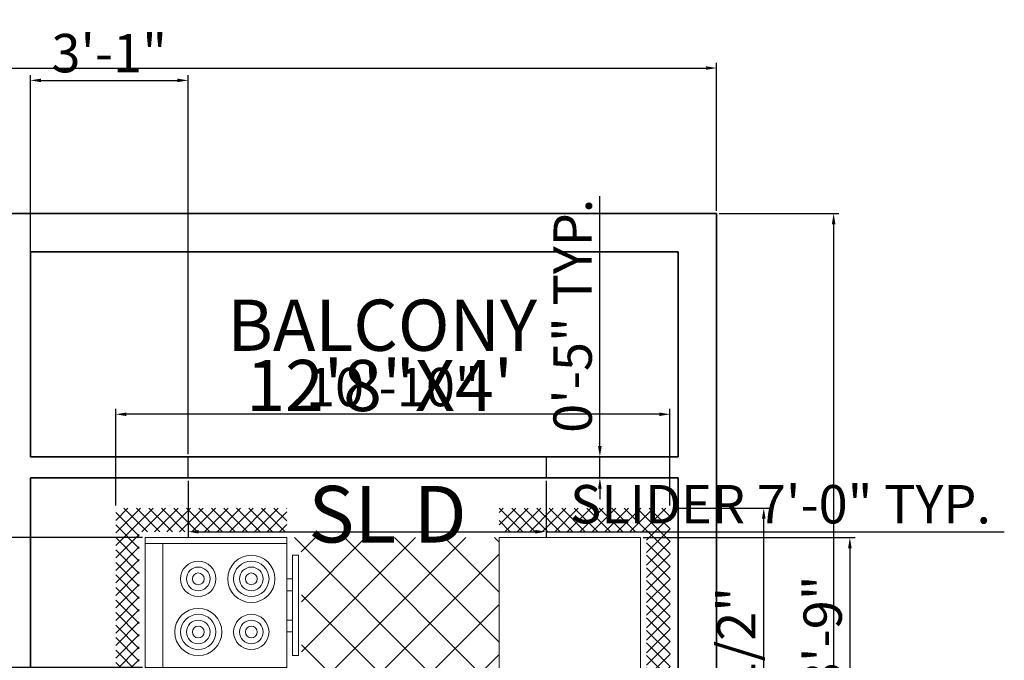
# Model space of a CAD drawing. Units: inches. Extents: x 3542 to 4275, y 1005 to 1722.
# Tile 6 of 6: x 4018 to 4249, y 1568 to 1718. Entities that reach past the tile are written whole.
import ezdxf

# ---------------------------------------------------------------- set-up
doc = ezdxf.new("R2010")
doc.units = ezdxf.units.IN
doc.layers.get('0').update_dxf_attribs({"color": 211})
for name, color, linetype, lineweight in [('A-ANNO-DIMS', 2, 'Continuous', 18), ('A-ANNO-TEXT', 7, 'Continuous', 18), ('A-AREA-IDEN', 7, 'Continuous', 25), ('A-DOOR', 3, 'Continuous', 25), ('A-FLOR-FIXT', 9, 'Continuous', 18), ('wall', 7, 'Continuous', 35)]:
    doc.layers.add(name, color=color, linetype=linetype, lineweight=lineweight)
doc.styles.get("Standard").update_dxf_attribs({"font": 'arial.ttf'})
doc.dimstyles.new('ISO-25', dxfattribs={"dimtxt": 9, "dimasz": 2.5, "dimexe": 1.25, "dimexo": 0.625, "dimtad": 1, "dimdec": 1, "dimlunit": 4, "dimtxsty": 'Standard', "dimcen": 2.5, "dimadec": 0, "dimazin": 0, "dimtfac": 1, "dimtdec": 1, "dimtmove": 0, "dimatfit": 3, "dimfxl": 1, "dimarcsym": 0})

# ---------------------------------------------------------------- blocks, each defined once
blk = doc.blocks.new('Kitchen Layout - 7 x 8 ft')
for p, q in [((-5, 81.32), (2.68, 89)), ((-5, 83.44), (0.56, 89)), ((-5, 85.56), (-1.56, 89)), ((-5, 87.68), (-3.68, 89)), ((-1, 84.97), (-5, 88.97)), ((1.09, 85), (-2.91, 89)), ((3.21, 85), (-0.79, 89)), ((0.81, 85), (4.81, 89)), ((5.34, 85), (1.34, 89)), ((2.93, 85), (6.93, 89)), ((7.46, 85), (3.46, 89)), ((5.05, 85), (9.05, 89)), ((9.58, 85), (5.58, 89)), ((7.17, 85), (11.17, 89)), ((11.7, 85), (7.7, 89)), ((9.29, 85), (13.29, 89)), ((13.82, 85), (9.82, 89)), ((11.41, 85), (15.41, 89)), ((15.94, 85), (11.94, 89)), ((13.53, 85), (17.53, 89)), ((18.06, 85), (14.06, 89)), ((15.65, 85), (19.65, 89)), ((20.18, 85), (16.18, 89)), ((17.78, 85), (21.78, 89)), ((22.31, 85), (18.31, 89)), ((19.9, 85), (23.9, 89)), ((24.43, 85), (20.43, 89)), ((22.02, 85), (26.02, 89)), ((26.55, 85), (22.55, 89)), ((24.14, 85), (28.14, 89)), ((28.67, 85), (24.67, 89)), ((26.26, 85), (30.26, 89)), ((30.79, 85), (26.79, 89)), ((28.38, 85), (32.38, 89)), ((32.91, 85), (28.91, 89)), ((30.5, 85), (34.5, 89)), ((35.03, 85), (31.03, 89)), ((32.63, 85), (36.63, 89)), ((37.16, 85), (33.16, 89)), ((34.75, 85), (38.75, 89)), ((39.28, 85), (35.28, 89)), ((36.87, 85), (40.87, 89)), ((41.4, 85), (37.4, 89)), ((38.99, 85), (42.99, 89)), ((43.52, 85), (39.52, 89)), ((41.11, 85), (45.11, 89)), ((45.64, 85), (41.64, 89)), ((43.23, 85), (47.23, 89)), ((47.76, 85), (43.76, 89)), ((45.35, 85), (49.35, 89)), ((49.88, 85), (45.88, 89)), ((47.47, 85), (51.47, 89)), ((52, 85), (48, 89)), ((49.6, 85), (53.6, 89)), ((54.13, 85), (50.13, 89)), ((51.72, 85), (55.72, 89)), ((56.25, 85), (52.25, 89)), ((53.84, 85), (57.84, 89)), ((58.37, 85), (54.37, 89)), ((55.96, 85), (59.96, 89)), ((60.49, 85), (56.49, 89)), ((58.08, 85), (62.08, 89)), ((62.61, 85), (58.61, 89)), ((60.2, 85), (64.2, 89)), ((64.73, 85), (60.73, 89)), ((62.32, 85), (66.32, 89)), ((66.85, 85), (62.85, 89)), ((64.45, 85), (68.45, 89)), ((68.97, 85), (64.97, 89)), ((66.57, 85), (70.57, 89)), ((71.1, 85), (67.1, 89)), ((68.69, 85), (72.69, 89)), ((73.22, 85), (69.22, 89)), ((70.81, 85), (74.81, 89)), ((75.34, 85), (71.34, 89)), ((72.93, 85), (76.93, 89)), ((77.46, 85), (73.46, 89)), ((75.05, 85), (79.05, 89)), ((79.58, 85), (75.58, 89)), ((77.17, 85), (81.17, 89)), ((81.7, 85), (77.7, 89)), ((79.29, 85), (83.29, 89)), ((83.82, 85), (79.82, 89)), ((81.42, 85), (85.42, 89)), ((85.95, 85), (81.95, 89)), ((83.54, 85), (87.54, 89)), ((88.07, 85), (84.07, 89)), ((85.66, 85), (89.66, 89)), ((90.19, 85), (86.19, 89)), ((87.78, 85), (91.78, 89)), ((92.31, 85), (88.31, 89)), ((89.9, 85), (93.9, 89)), ((94.43, 85), (90.43, 89)), ((92.02, 85), (96.02, 89)), ((96.55, 85), (92.55, 89)), ((94.14, 85), (98.14, 89)), ((101, 82.67), (94.67, 89)), ((96.27, 85), (100.27, 89)), ((101, 84.79), (96.79, 89)), ((101, 86.92), (98.92, 89)), ((-1, 82.85), (-5, 86.85)), ((97, 83.61), (101, 87.61)), ((97, 81.49), (101, 85.49)), ((-1, 80.73), (-5, 84.73)), ((34, 84), (96, 84)), ((34, 60), (34, 84)), ((96, 84), (96, 60)), ((101, 80.55), (97, 84.55)), ((-5, 79.19), (-1, 83.19)), ((-1, 78.61), (-5, 82.61)), ((97, 79.37), (101, 83.37)), ((101, 78.43), (97, 82.43)), ((-5, 77.07), (-1, 81.07)), ((-1, 76.49), (-5, 80.49)), ((74, 81), (95, 81)), ((97, 77.25), (101, 81.25)), ((101, 76.31), (97, 80.31)), ((-5, 74.95), (-1, 78.95)), ((97, 75.13), (101, 79.13)), ((-1, 74.36), (-5, 78.36)), ((-5, 72.83), (-1, 76.83)), ((101, 74.19), (97, 78.19)), ((97, 73.01), (101, 77.01)), ((-1, 72.24), (-5, 76.24)), ((101, 72.07), (97, 76.07)), ((-5, 70.71), (-1, 74.71)), ((-1, 70.12), (-5, 74.12)), ((97, 70.89), (101, 74.89)), ((101, 69.95), (97, 73.95)), ((-5, 68.59), (-1, 72.59)), ((-1, 68), (-5, 72)), ((97, 68.76), (101, 72.76)), ((101, 67.82), (97, 71.82)), ((-5, 66.47), (-1, 70.47)), ((97, 66.64), (101, 70.64)), ((-1, 65.88), (-5, 69.88)), ((101, 65.7), (97, 69.7)), ((97, 64.52), (101, 68.52)), ((-5, 64.35), (-1, 68.35)), ((-1, 63.76), (-5, 67.76)), ((101, 63.58), (97, 67.58)), ((-5, 62.22), (-1, 66.22)), ((-1, 61.64), (-5, 65.64)), ((97, 62.4), (101, 66.4)), ((101, 61.46), (97, 65.46)), ((-5, 60.1), (-1, 64.1)), ((-1, 59.52), (-5, 63.52)), ((97, 60.28), (101, 64.28)), ((-5, 57.98), (-1, 61.98)), ((100.34, 60), (97, 63.34)), ((98.84, 60), (101, 62.16)), ((-1, 57.39), (-5, 61.39)), ((98.22, 60), (97, 61.22)), ((-1.73, 56), (-5, 59.27)), ((-4.86, 56), (-1, 59.86)), ((10.4, 24), (45.9, 59.5)), ((18.88, 24), (54.38, 59.5)), ((27.37, 24), (62.87, 59.5)), ((33.03, 55.11), (37.41, 59.5)), ((96, 60), (34, 60)), ((35.85, 24), (71.35, 59.5)), ((76.2, 24), (40.7, 59.5)), ((84.68, 24), (49.18, 59.5)), ((93.17, 24), (57.67, 59.5)), ((61.31, 24), (96, 58.69)), ((96, 29.65), (66.15, 59.5)), ((80, 60), (80, 59)), ((82, 59), (82, 60)), ((87, 59), (87, 60)), ((89, 60), (89, 59)), ((100.96, 60), (101, 60.04)), ((-3.85, 56), (-5, 57.15)), ((-2.74, 56), (-1, 57.74)), ((0, 57), (33, 57)), ((67.71, 24), (33.68, 58.04)), ((44.34, 24), (77.84, 57.5)), ((52.82, 24), (86.32, 57.5)), ((96, 38.14), (76.64, 57.5)), ((96, 46.63), (85.13, 57.5)), ((96, 55.11), (93.57, 57.54)), ((31, 55), (31, 56)), ((32, 56), (32, 55)), ((0, 30.57), (24.43, 55)), ((0, 39.06), (15.94, 55)), ((0, 47.54), (7.46, 55)), ((1.91, 24), (32.91, 55)), ((33.77, 24), (2.77, 55)), ((42.26, 24), (11.26, 55)), ((50.74, 24), (19.74, 55)), ((59.23, 24), (28.23, 55)), ((32, 55), (31, 55)), ((69.79, 24), (96, 50.21)), ((25.29, 24), (0, 49.29)), ((16.8, 24), (0, 40.8)), ((78.28, 24), (96, 41.72)), ((8.32, 24), (0, 32.32)), ((86.76, 24), (96, 33.24)), ((-5, 21.92), (-2.92, 24)), ((-5, 19.8), (-1, 23.8)), ((-1, 21.33), (-3.67, 24)), ((-1, 23.45), (-1.55, 24)), ((0, 24), (96, 24)), ((0, 0), (0, 24)), ((95.25, 24), (96, 24.75)), ((96, 24), (96, 0)), ((97, 22.1), (98.9, 24)), ((97, 19.97), (101, 23.97)), ((101, 21.16), (98.16, 24)), ((101, 23.28), (100.28, 24)), ((-1, 19.21), (-5, 23.21)), ((101, 19.03), (97, 23.03)), ((97, 17.85), (101, 21.85)), ((-5, 17.68), (-1, 21.68)), ((-1, 17.09), (-5, 21.09)), ((101, 16.91), (97, 20.91)), ((-5, 15.55), (-1, 19.55)), ((-1, 14.97), (-5, 18.97)), ((47.25, 6.5), (47.25, 18.5)), ((48.75, 18.5), (48.75, 6.5)), ((97, 15.73), (101, 19.73)), ((101, 14.79), (97, 18.79)), ((-5, 13.43), (-1, 17.43)), ((-1, 12.85), (-5, 16.85)), ((97, 13.61), (101, 17.61)), ((-5, 11.31), (-1, 15.31)), ((101, 12.67), (97, 16.67)), ((97, 11.49), (101, 15.49)), ((-1, 10.73), (-5, 14.73)), ((101, 10.55), (97, 14.55)), ((97, 9.37), (101, 13.37)), ((-5, 9.19), (-1, 13.19)), ((-1, 8.6), (-5, 12.6)), ((101, 8.43), (97, 12.43)), ((-5, 7.07), (-1, 11.07)), ((-1, 6.48), (-5, 10.48)), ((97, 7.25), (101, 11.25)), ((101, 6.31), (97, 10.31)), ((-5, 4.95), (-1, 8.95)), ((-1, 4.36), (-5, 8.36)), ((97, 5.12), (101, 9.12)), ((-5, 2.83), (-1, 6.83)), ((101, 4.18), (97, 8.18)), ((97, 3), (101, 7)), ((-1, 2.24), (-5, 6.24)), ((101, 2.06), (97, 6.06)), ((-5, 0.71), (-1, 4.71)), ((-1, 0.12), (-5, 4.12)), ((64, 4), (32, 4)), ((97, 0.88), (101, 4.88)), ((101, -0.06), (97, 3.94)), ((-5, -1.42), (-1, 2.58)), ((2, -5), (-5, 2)), ((93.24, -5), (101, 2.76)), ((101, -2.18), (97, 1.82)), ((-5, -3.54), (-1, 0.46)), ((96, 0), (0, 0)), ((95.36, -5), (101, 0.64)), ((-0.12, -5), (-5, -0.12)), ((-4.34, -5), (-0.34, -1)), ((-2.22, -5), (1.78, -1)), ((-0.1, -5), (3.9, -1)), ((4.12, -5), (0.12, -1)), ((2.02, -5), (6.02, -1)), ((6.24, -5), (2.24, -1)), ((4.14, -5), (8.14, -1)), ((8.36, -5), (4.36, -1)), ((6.27, -5), (10.27, -1)), ((10.48, -5), (6.48, -1)), ((8.39, -5), (12.39, -1)), ((12.6, -5), (8.6, -1)), ((10.51, -5), (14.51, -1)), ((14.73, -5), (10.73, -1)), ((12.63, -5), (16.63, -1)), ((16.85, -5), (12.85, -1)), ((14.75, -5), (18.75, -1)), ((18.97, -5), (14.97, -1)), ((16.87, -5), (20.87, -1)), ((21.09, -5), (17.09, -1)), ((18.99, -5), (22.99, -1)), ((23.21, -5), (19.21, -1)), ((21.11, -5), (25.11, -1)), ((25.33, -5), (21.33, -1)), ((23.24, -5), (27.24, -1)), ((27.45, -5), (23.45, -1)), ((25.36, -5), (29.36, -1)), ((29.57, -5), (25.57, -1)), ((30, -3.3), (27.7, -1)), ((30, -1.18), (29.82, -1)), ((66, -2.54), (67.54, -1)), ((66, -4.66), (69.66, -1)), ((69.88, -5), (66, -1.12)), ((67.78, -5), (71.78, -1)), ((72, -5), (68, -1)), ((69.9, -5), (73.9, -1)), ((74.12, -5), (70.12, -1)), ((72.03, -5), (76.03, -1)), ((76.24, -5), (72.24, -1)), ((74.15, -5), (78.15, -1)), ((78.36, -5), (74.36, -1)), ((76.27, -5), (80.27, -1)), ((80.49, -5), (76.49, -1)), ((78.39, -5), (82.39, -1)), ((82.61, -5), (78.61, -1)), ((80.51, -5), (84.51, -1)), ((84.73, -5), (80.73, -1)), ((82.63, -5), (86.63, -1)), ((86.85, -5), (82.85, -1)), ((84.75, -5), (88.75, -1)), ((88.97, -5), (84.97, -1)), ((86.88, -5), (90.88, -1)), ((91.09, -5), (87.09, -1)), ((89, -5), (93, -1)), ((93.21, -5), (89.21, -1)), ((91.12, -5), (95.12, -1)), ((95.34, -5), (91.34, -1)), ((97.46, -5), (93.46, -1)), ((99.58, -5), (95.58, -1)), ((101, -4.3), (97, -0.3)), ((97.48, -5), (101, -1.48)), ((-2.25, -5), (-5, -2.25)), ((27.48, -5), (30, -2.48)), ((67.76, -5), (66, -3.24)), ((-4.37, -5), (-5, -4.37)), ((29.6, -5), (30, -4.6)), ((99.6, -5), (101, -3.6))]:
    blk.add_line(p, q)
for points in [[(0, 56), (0, 84), (33, 84), (33, 56)], [(74, 60), (74, 84), (95, 84), (95, 60)], [(76, 58), (76, 59), (93, 59), (93, 58)]]:
    blk.add_lwpolyline(points, close=True)
for points in [[(33.5, 21), (62.5, 21)], [(32, 1.5), (32, 19.5)], [(33.5, 6.5), (33.5, 18.5)], [(34.5, 19.5), (46.25, 19.5)], [(49.75, 19.5), (61.5, 19.5)], [(62.5, 18.5), (62.5, 6.5)], [(64, 19.5), (64, 1.5)], [(46.25, 5.5), (34.5, 5.5)], [(61.5, 5.5), (49.75, 5.5)], [(62.5, 0), (33.5, 0)]]:
    blk.add_lwpolyline(points)
for centre, radius in [((80, 75), 4), ((80, 75), 3), ((80, 75), 2), ((89, 75), 3), ((89, 75), 2), ((80, 75), 1), ((89, 75), 1), ((80, 66), 3), ((89, 66), 4), ((89, 66), 3), ((80, 66), 2), ((80, 66), 1), ((89, 66), 2), ((89, 66), 1), ((40.5, 12.5), 1), ((55.5, 12.5), 1), ((40.5, 12.5), 0.5), ((55.5, 12.5), 0.5)]:
    blk.add_circle(centre, radius)
for centre, radius, start, end in [((33.5, 19.5), 1.5, 90, 180), ((62.5, 19.5), 1.5, 0, 90), ((34.5, 18.5), 1, 90, 180), ((46.25, 18.5), 1, 0, 90), ((49.75, 18.5), 1, 90, 180), ((61.5, 18.5), 1, 0, 90), ((34.5, 6.5), 1, 180, 270), ((46.25, 6.5), 1, 270, 0), ((49.75, 6.5), 1, 180, 270), ((61.5, 6.5), 1, 270, 0), ((33.5, 1.5), 1.5, 180, 270), ((62.5, 1.5), 1.5, 270, 0)]:
    blk.add_arc(centre, radius, start, end)
blk = doc.blocks.new('*D12')
at = {"layer": 'A-ANNO-DIMS', "color": 0, "lineweight": -2, "transparency": 16777216}
for p, q in [((3641.89, 1673.05), (3641.89, 1707.82)), ((4181.89, 1673.05), (4181.89, 1707.82)), ((3644.39, 1706.57), (4179.39, 1706.57))]:
    blk.add_line(p, q, dxfattribs=at)
at = {"layer": 'A-ANNO-DIMS', "color": 0, "transparency": 16777216}
for points in [[(3644.39, 1706.99), (3644.39, 1706.16), (3641.89, 1706.57)], [(4179.39, 1706.99), (4179.39, 1706.16), (4181.89, 1706.57)]]:
    blk.add_solid(points, dxfattribs=at)
at = {"layer": 'Defpoints', "color": 0, "transparency": 16777216}
for p in [(4181.89, 1706.57), (3641.89, 1672.43), (4181.89, 1672.43)]:
    blk.add_point(p, dxfattribs=at)
at = {"layer": 'A-ANNO-DIMS', "color": 0, "transparency": 16777216, "insert": (3911.89, 1711.77), "char_height": 9, "attachment_point": 5}
blk.add_mtext("45'", dxfattribs=at)
blk = doc.blocks.new('*D13')
at = {"layer": 'A-ANNO-DIMS', "color": 0, "lineweight": -2, "transparency": 16777216}
for p, q in [((4182.51, 1672.43), (4210.58, 1672.43)), ((4209.33, 1669.93), (4209.33, 1134.93)), ((4182.51, 1132.43), (4210.58, 1132.43))]:
    blk.add_line(p, q, dxfattribs=at)
at = {"layer": 'A-ANNO-DIMS', "color": 0, "transparency": 16777216}
for points in [[(4208.91, 1669.93), (4209.75, 1669.93), (4209.33, 1672.43)], [(4208.91, 1134.93), (4209.75, 1134.93), (4209.33, 1132.43)]]:
    blk.add_solid(points, dxfattribs=at)
at = {"layer": 'Defpoints', "color": 0, "transparency": 16777216}
for p in [(4181.89, 1672.43), (4181.89, 1132.43), (4209.33, 1132.43)]:
    blk.add_point(p, dxfattribs=at)
at = {"layer": 'A-ANNO-DIMS', "color": 0, "transparency": 16777216, "insert": (4204.13, 1402.43), "char_height": 9, "attachment_point": 5, "rotation": 90}
blk.add_mtext("45'", dxfattribs=at)
blk = doc.blocks.new('DOOR-SLIDING-84IN')
blk.add_lwpolyline([(0, 0), (0, 5), (84, 5), (84, 0)], close=True)
blk = doc.blocks.new('*D21')
at = {"layer": 'A-ANNO-DIMS', "color": 0, "lineweight": -2, "transparency": 16777216}
for p, q in [((4057.89, 1609.8), (4057.89, 1596.58)), ((4141.89, 1609.8), (4141.89, 1596.58)), ((4060.39, 1597.83), (4139.39, 1597.83)), ((4141.89, 1597.83), (4249.37, 1597.83))]:
    blk.add_line(p, q, dxfattribs=at)
at = {"layer": 'A-ANNO-DIMS', "color": 0, "transparency": 16777216}
for points in [[(4060.39, 1598.24), (4060.39, 1597.41), (4057.89, 1597.83)], [(4139.39, 1598.24), (4139.39, 1597.41), (4141.89, 1597.83)]]:
    blk.add_solid(points, dxfattribs=at)
at = {"layer": 'Defpoints', "color": 0, "transparency": 16777216}
for p in [(4057.89, 1610.43), (4141.89, 1610.43), (4141.89, 1597.83)]:
    blk.add_point(p, dxfattribs=at)
at = {"layer": 'A-ANNO-DIMS', "color": 0, "transparency": 16777216, "insert": (4196.88, 1603.11), "char_height": 9, "attachment_point": 5}
blk.add_mtext('SLIDER 7\'-0" TYP.', dxfattribs=at)
blk = doc.blocks.new('*D22')
at = {"layer": 'A-ANNO-DIMS', "color": 0, "lineweight": -2, "transparency": 16777216}
for p, q in [((4154.49, 1617.93), (4154.49, 1676.54)), ((4142.52, 1615.43), (4155.74, 1615.43)), ((4154.49, 1610.43), (4154.49, 1615.43)), ((4142.52, 1610.43), (4155.74, 1610.43)), ((4154.49, 1607.93), (4154.49, 1605.43))]:
    blk.add_line(p, q, dxfattribs=at)
at = {"layer": 'A-ANNO-DIMS', "color": 0, "transparency": 16777216}
for points in [[(4154.07, 1617.93), (4154.91, 1617.93), (4154.49, 1615.43)], [(4154.07, 1607.93), (4154.91, 1607.93), (4154.49, 1610.43)]]:
    blk.add_solid(points, dxfattribs=at)
at = {"layer": 'Defpoints', "color": 0, "transparency": 16777216}
for p in [(4141.89, 1615.43), (4154.49, 1615.43), (4141.89, 1610.43)]:
    blk.add_point(p, dxfattribs=at)
at = {"layer": 'A-ANNO-DIMS', "color": 0, "transparency": 16777216, "insert": (4149.27, 1648.48), "char_height": 9, "attachment_point": 5, "rotation": 90}
blk.add_mtext('0\'-5" TYP.', dxfattribs=at)
blk = doc.blocks.new('*D27')
at = {"layer": 'A-ANNO-DIMS', "color": 0, "lineweight": -2, "transparency": 16777216}
for p, q in [((4171.57, 1603.37), (4194.19, 1603.37)), ((4192.94, 1459.24), (4192.94, 1600.87)), ((4171.57, 1456.74), (4194.19, 1456.74))]:
    blk.add_line(p, q, dxfattribs=at)
at = {"layer": 'A-ANNO-DIMS', "color": 0, "transparency": 16777216}
for points in [[(4192.52, 1600.87), (4193.36, 1600.87), (4192.94, 1603.37)], [(4192.52, 1459.24), (4193.36, 1459.24), (4192.94, 1456.74)]]:
    blk.add_solid(points, dxfattribs=at)
at = {"layer": 'Defpoints', "color": 0, "transparency": 16777216}
for p in [(4170.94, 1603.37), (4192.94, 1603.37), (4170.94, 1456.74)]:
    blk.add_point(p, dxfattribs=at)
at = {"layer": 'A-ANNO-DIMS', "color": 0, "transparency": 16777216, "insert": (4187.66, 1530.06), "char_height": 9, "attachment_point": 5, "rotation": 90}
blk.add_mtext('KITCHEN 12\'-2 1/2"', dxfattribs=at)
blk = doc.blocks.new('*D28')
at = {"layer": 'A-ANNO-DIMS', "color": 0, "lineweight": -2, "transparency": 16777216}
for p, q in [((4040.91, 1604), (4040.91, 1626.62)), ((4170.94, 1604), (4170.94, 1626.62)), ((4168.44, 1625.37), (4043.41, 1625.37))]:
    blk.add_line(p, q, dxfattribs=at)
at = {"layer": 'A-ANNO-DIMS', "color": 0, "transparency": 16777216}
for points in [[(4043.41, 1625.79), (4043.41, 1624.95), (4040.91, 1625.37)], [(4168.44, 1625.79), (4168.44, 1624.95), (4170.94, 1625.37)]]:
    blk.add_solid(points, dxfattribs=at)
at = {"layer": 'Defpoints', "color": 0, "transparency": 16777216}
for p in [(4040.91, 1625.37), (4040.91, 1603.37), (4170.94, 1603.37)]:
    blk.add_point(p, dxfattribs=at)
at = {"layer": 'A-ANNO-DIMS', "color": 0, "transparency": 16777216, "insert": (4105.93, 1630.59), "char_height": 9, "attachment_point": 5}
blk.add_mtext('10\'-10"', dxfattribs=at)
blk = doc.blocks.new('*D44')
at = {"layer": 'A-ANNO-DIMS', "color": 0, "lineweight": -2, "transparency": 16777216}
for p, q in [((4020.89, 1616.05), (4020.89, 1704.93)), ((4057.89, 1616.05), (4057.89, 1704.93)), ((4023.39, 1703.68), (4055.39, 1703.68))]:
    blk.add_line(p, q, dxfattribs=at)
at = {"layer": 'A-ANNO-DIMS', "color": 0, "transparency": 16777216}
for points in [[(4023.39, 1704.09), (4023.39, 1703.26), (4020.89, 1703.68)], [(4055.39, 1704.09), (4055.39, 1703.26), (4057.89, 1703.68)]]:
    blk.add_solid(points, dxfattribs=at)
at = {"layer": 'Defpoints', "color": 0, "transparency": 16777216}
for p in [(4057.89, 1703.68), (4020.89, 1615.43), (4057.89, 1615.43)]:
    blk.add_point(p, dxfattribs=at)
at = {"layer": 'A-ANNO-DIMS', "color": 0, "transparency": 16777216, "insert": (4039.39, 1708.9), "char_height": 9, "attachment_point": 5}
blk.add_mtext('3\'-1"', dxfattribs=at)
blk = doc.blocks.new('*D54')
at = {"layer": 'A-ANNO-DIMS', "color": 0, "lineweight": -2, "transparency": 16777216}
for p, q in [((4047.2, 1596.46), (3559.02, 1596.46)), ((3560.27, 1593.96), (3560.27, 1568.52)), ((4047.2, 1566.02), (3559.02, 1566.02)), ((3560.27, 1566.02), (3560.27, 1517.22))]:
    blk.add_line(p, q, dxfattribs=at)
at = {"layer": 'A-ANNO-DIMS', "color": 0, "transparency": 16777216}
for points in [[(3559.85, 1593.96), (3560.69, 1593.96), (3560.27, 1596.46)], [(3559.85, 1568.52), (3560.69, 1568.52), (3560.27, 1566.02)]]:
    blk.add_solid(points, dxfattribs=at)
at = {"layer": 'Defpoints', "color": 0, "transparency": 16777216}
for p in [(4047.82, 1596.46), (3560.27, 1566.02), (4047.82, 1566.02)]:
    blk.add_point(p, dxfattribs=at)
at = {"layer": 'A-ANNO-DIMS', "color": 0, "transparency": 16777216, "insert": (3554.99, 1540.37), "char_height": 9, "attachment_point": 5, "rotation": 90}
blk.add_mtext('2\'-6 1/2"', dxfattribs=at)
blk = doc.blocks.new('*D58')
at = {"layer": 'A-ANNO-DIMS', "color": 0, "lineweight": -2, "transparency": 16777216}
for p, q in [((4164.65, 1596.46), (4214.39, 1596.46)), ((4213.14, 1593.96), (4213.14, 1554.08)), ((4164.04, 1551.58), (4214.39, 1551.58))]:
    blk.add_line(p, q, dxfattribs=at)
at = {"layer": 'A-ANNO-DIMS', "color": 0, "transparency": 16777216}
for points in [[(4212.72, 1593.96), (4213.56, 1593.96), (4213.14, 1596.46)], [(4212.72, 1554.08), (4213.56, 1554.08), (4213.14, 1551.58)]]:
    blk.add_solid(points, dxfattribs=at)
at = {"layer": 'Defpoints', "color": 0, "transparency": 16777216}
for p in [(4164.03, 1596.46), (4163.42, 1551.58), (4213.14, 1551.58)]:
    blk.add_point(p, dxfattribs=at)
at = {"layer": 'A-ANNO-DIMS', "color": 0, "transparency": 16777216, "insert": (4207.92, 1574.02), "char_height": 9, "attachment_point": 5, "rotation": 90}
blk.add_mtext('3\'-9"', dxfattribs=at)

msp = doc.modelspace()

# ---------------------------------------------------------------- linework, layer by layer
at = {"layer": 'wall'}
for p, q in [((3641.89, 1672.43), (4181.89, 1672.43)), ((4181.89, 1672.43), (4181.89, 1132.43)), ((4020.89, 1663.43), (4172.89, 1663.43)), ((4020.89, 1615.43), (4020.89, 1663.43)), ((4172.89, 1663.43), (4172.89, 1615.43)), ((4020.89, 1615.43), (4172.89, 1615.43)), ((4020.89, 1448.43), (4020.89, 1610.43)), ((4020.89, 1610.43), (4172.89, 1610.43)), ((4172.89, 1610.43), (4172.89, 1448.43))]:
    msp.add_line(p, q, dxfattribs=at)

# ---------------------------------------------------------------- block references
at = {"layer": 'A-DOOR'}
msp.add_blockref('DOOR-SLIDING-84IN', (4057.89, 1610.43), dxfattribs=at)
at = {"layer": 'A-FLOR-FIXT', "xscale": 1.383356761737284, "yscale": 1.383356761737284, "zscale": 1.383356761737284, "rotation": 90}
msp.add_blockref('Kitchen Layout - 7 x 8 ft', (4164.03, 1463.65), dxfattribs=at)

# ---------------------------------------------------------------- texts
at = {"layer": 'A-ANNO-TEXT'}
msp.add_text('SL D', height=13.276, dxfattribs=at).set_placement((4086.11, 1595.3))
at = {"layer": 'A-AREA-IDEN'}
for s, p in [('BALCONY', (4067.05, 1640.25)), ('12\'8"X4\'', (4071.55, 1626.12))]:
    msp.add_text(s, height=12, dxfattribs=at).set_placement(p)

# ---------------------------------------------------------------- dimensions: what is measured, and where the dimension line sits
at = {"layer": 'A-ANNO-DIMS'}
for base, p1, p2, override, picture, middle in [((4181.89, 1706.57), (3641.89, 1672.43), (4181.89, 1672.43), {"dimclrd": 0, "dimclre": 0, "dimclrt": 0}, '*D12', (3911.89, 1711.77)), ((4057.89, 1703.68), (4020.89, 1615.43), (4057.89, 1615.43), {"dimdec": 1, "dimlfac": 1, "dimrnd": 0, "dimzin": 1, "dimdsep": 46, "dimlunit": 4, "dimfrac": 2}, '*D44', (4039.39, 1708.9))]:
    dim = msp.add_linear_dim(base=base, p1=p1, p2=p2, dimstyle='ISO-25', override=override, dxfattribs=at)
    dim.commit()
    dim.dimension.update_dxf_attribs({"geometry": picture, "text_midpoint": middle})
for base, p1, p2, text, picture, middle in [((4154.49, 1615.43), (4141.89, 1610.43), (4141.89, 1615.43), '<> TYP.', '*D22', (4149.27, 1648.48)), ((4192.94, 1603.37), (4170.94, 1456.74), (4170.94, 1603.37), 'KITCHEN <>', '*D27', (4187.66, 1530.06))]:
    dim = msp.add_linear_dim(base=base, p1=p1, p2=p2, angle=90, text=text, dimstyle='ISO-25', override={"dimdec": 1, "dimlfac": 1, "dimrnd": 0, "dimzin": 1, "dimdsep": 46, "dimlunit": 4, "dimfrac": 2}, dxfattribs=at)
    dim.commit()
    dim.dimension.update_dxf_attribs({"geometry": picture, "text_midpoint": middle})
for base, p1, p2, angle, override, picture, middle in [((4209.33, 1132.43), (4181.89, 1672.43), (4181.89, 1132.43), 90, {"dimclrd": 0, "dimclre": 0, "dimclrt": 0}, '*D13', (4204.13, 1402.43)), ((4040.91, 1625.37), (4170.94, 1603.37), (4040.91, 1603.37), 180, {"dimdec": 1, "dimlfac": 1, "dimrnd": 0, "dimzin": 1, "dimdsep": 46, "dimlunit": 4, "dimfrac": 2}, '*D28', (4105.93, 1630.59)), ((3560.27, 1566.02), (4047.82, 1596.46), (4047.82, 1566.02), 90, {"dimdec": 1, "dimlfac": 1, "dimrnd": 0, "dimzin": 1, "dimdsep": 46, "dimlunit": 4, "dimfrac": 2}, '*D54', (3554.99, 1540.37)), ((4213.14, 1551.58), (4164.03, 1596.46), (4163.42, 1551.58), 90, {"dimdec": 1, "dimlfac": 1, "dimrnd": 0, "dimzin": 1, "dimdsep": 46, "dimlunit": 4, "dimfrac": 2}, '*D58', (4207.92, 1574.02))]:
    dim = msp.add_linear_dim(base=base, p1=p1, p2=p2, angle=angle, dimstyle='ISO-25', override=override, dxfattribs=at)
    dim.commit()
    dim.dimension.update_dxf_attribs({"geometry": picture, "text_midpoint": middle})
dim = msp.add_linear_dim(base=(4141.89, 1597.83), p1=(4057.89, 1610.43), p2=(4141.89, 1610.43), text='SLIDER <> TYP.', dimstyle='ISO-25', override={"dimdec": 1, "dimlfac": 1, "dimrnd": 0, "dimzin": 1, "dimdsep": 46, "dimlunit": 4, "dimfrac": 2}, dxfattribs=at)
dim.commit()
dim.dimension.update_dxf_attribs({"geometry": '*D21', "text_midpoint": (4196.88, 1603.11)})

doc.saveas('drawing.dxf')
